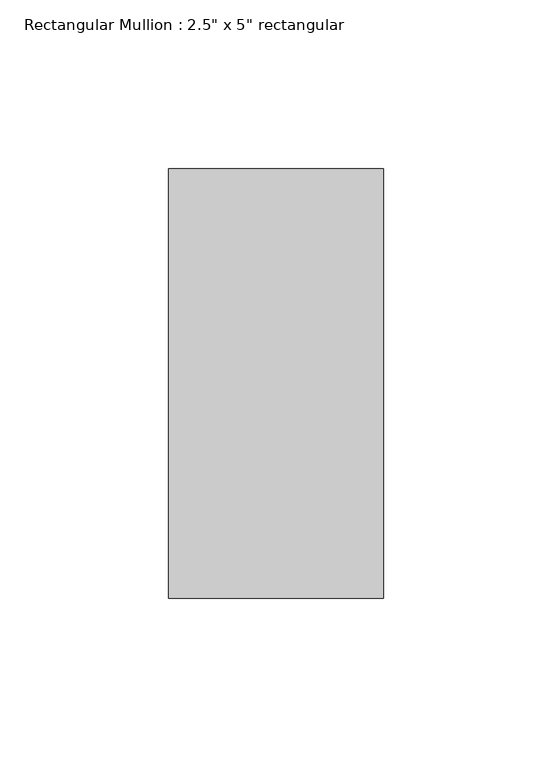
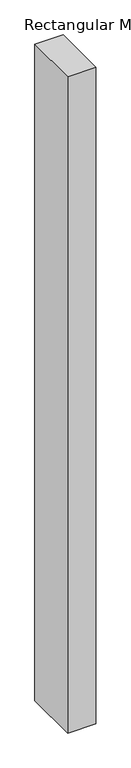
"""IFC4 building model written with IfcOpenShell, lengths in millimetres: member geometry."""

from ifc_helpers import new_model, si_unit, frame, origin, place, context, project, spatial, polyline, outline, extrude, source, transform, mapped, element, save


def member_973bd760(model_context):
    return source(origin(), model_context, "Body", "SweptSolid", [
        extrude(outline(polyline([(0.0, 63.5), (0.0, -63.5), (-63.5, -63.5), (-63.5, 63.5), (0.0, 63.5)])), frame((0.0, 0.0, -1560.9513331), z_axis=(0.0, 0.0, 1.0), x_axis=(1.0, 0.0, 0.0)), (0.0, 0.0, 1.0), 1560.9513331),
    ])


if __name__ == "__main__":
    model = new_model("IFC4")
    model_context = context("Model", 3, world=origin())
    ifc_project = project(units=[si_unit("LENGTHUNIT", "METRE", prefix="MILLI")], contexts=[model_context])
    site = spatial("IfcSite", under=ifc_project)
    building = spatial("IfcBuilding", under=site)
    placement = place(None, origin())
    member_shape = member_973bd760(model_context)
    element("IfcMember", 1, ObjectType="Rectangular Mullion : 2.5\" x 5\" rectangular", at=placement, inside=building, context=model_context, shape_type="MappedRepresentation", body=[
        mapped(member_shape, transform((0.0, 0.0, 0.0), x_axis=(1.0, 0.0, 0.0), y_axis=(0.0, 1.0, 0.0), z_axis=(0.0, 0.0, 1.0))),
    ])
    save(model, "model.ifc")

# Revit data of these elements
# Type "Rectangular Mullion : 2.5\" x 5\" rectangular"
#   built-in parameter 1007304 = 0.416667 (stored number, unit not read)
#   built-in parameter 1007301 = 0.104167 (stored number, unit not read)
#   built-in parameter 1007300 = 0.104167 (stored number, unit not read)
# Element 1 (IfcMember, "Rectangular Mullion : 2.5\" x 5\" rectangular")
#   Materials on its faces: "Aluminum"
# Materials
#   "Aluminum": class "Metal", colour RGB 247 247 247, transparency 0, Description = "Aluminum 6061", Cost = 0
